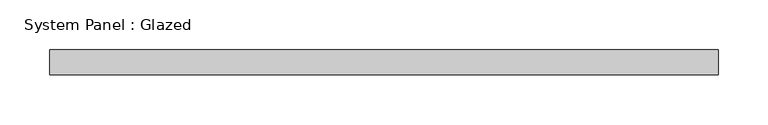
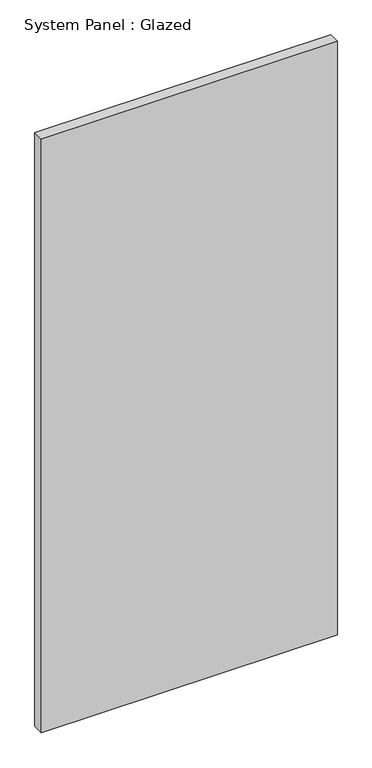
"""IFC4 building model written with IfcOpenShell, lengths in millimetres: plate geometry, System Panel : Glazed."""

from ifc_helpers import new_model, si_unit, origin, origin_with_axes, place, context, project, spatial, polyline, outline, extrude, source, transform, mapped, element, save


def system_panel_glazed_f5076819(model_context):
    return source(origin(), model_context, "Body", "SweptSolid", [
        extrude(outline(polyline([(336.55, 19.05), (-336.55, 19.05), (-336.55, 44.45), (336.55, 44.45), (336.55, 19.05)])), origin_with_axes(), (0.0, 0.0, 1.0), 1426.5106693),
    ])


if __name__ == "__main__":
    model = new_model("IFC4")
    model_context = context("Model", 3, world=origin())
    ifc_project = project(units=[si_unit("LENGTHUNIT", "METRE", prefix="MILLI")], contexts=[model_context])
    site = spatial("IfcSite", under=ifc_project)
    building = spatial("IfcBuilding", under=site)
    placement = place(None, origin())
    system_panel_glazed_shape = system_panel_glazed_f5076819(model_context)
    element("IfcPlate", 1, ObjectType="System Panel : Glazed", at=placement, inside=building, context=model_context, shape_type="MappedRepresentation", body=[
        mapped(system_panel_glazed_shape, transform((0.0, 0.0, 0.0), x_axis=(1.0, 0.0, 0.0), y_axis=(0.0, 1.0, 0.0), z_axis=(0.0, 0.0, 1.0))),
    ])
    save(model, "model.ifc")

# Revit data of these elements
# Type "System Panel : Glazed"
#   Construction Type Id = "GSP4R"
#   Analytic Construction = "1/8 in Pilkington single glazing"
#   Visual Light Transmittance = 0.9
#   Solar Heat Gain Coefficient = 0.86
#   Heat Transfer Coefficient (U) = 1.18115 BTU/(h·ft²·°F)
#   Define Thermal Properties by = 1
# Element 1 (IfcPlate, "System Panel : Glazed")
#   Materials on its faces: "Glass"
# Materials
#   "Glass": class "Glass", colour RGB 0 128 192, transparency 0.75, Description = "Soda Lime Glass", Cost = 0
